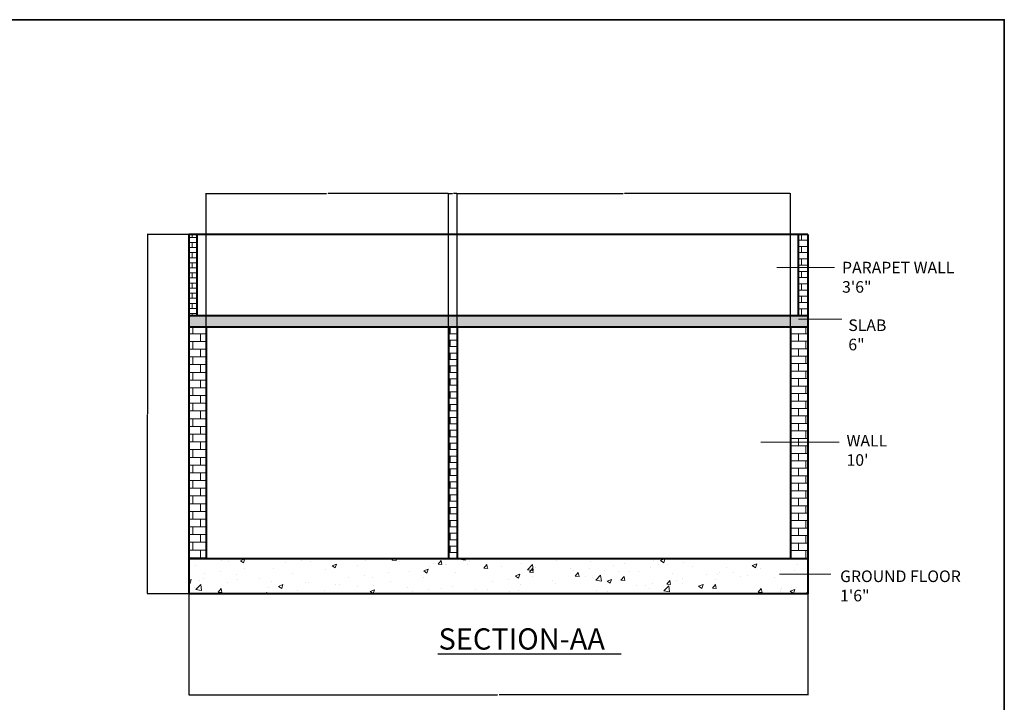
# Model space of a CAD drawing. Units: inches. Extents: x 1441 to 2460, y 1648 to 2683.
# Tile 35 of 35: x 1950 to 2460, y 2329 to 2683. Entities that reach past the tile are written whole.
import ezdxf

# ---------------------------------------------------------------- set-up
doc = ezdxf.new("R2010")
doc.units = ezdxf.units.IN
for name, color, linetype, lineweight in [('A-ANNO-DIMS', 2, 'Continuous', 18), ('A-ANNO-TEXT', 7, 'Continuous', 18), ('A-ANNO-TITL', 7, 'Continuous', 30), ('A-ANNO-TTLB', 7, 'Continuous', 35), ('A-SECT', 7, 'Continuous', 40)]:
    doc.layers.add(name, color=color, linetype=linetype, lineweight=lineweight)
doc.layers.add('A-SECT-PATT', color=251, linetype='Continuous', lineweight=13, true_color=0x636466)
doc.styles.get("Standard").update_dxf_attribs({"font": 'arial.ttf'})
doc.dimstyles.get("Standard").update_dxf_attribs({"dimtxt": 0.18, "dimasz": 0.18, "dimexe": 0.18, "dimexo": 0.0625, "dimgap": 0.09, "dimtad": 0, "dimtih": 1, "dimtoh": 1, "dimdec": 4, "dimzin": 0, "dimdsep": 46, "dimtxsty": 'Standard', "dimcen": 0.09, "dimadec": 0, "dimazin": 0, "dimtfac": 1, "dimtdec": 4, "dimtofl": 0, "dimtmove": 0, "dimatfit": 3, "dimfxl": 1, "dimtolj": 1, "dimtzin": 0, "dimarcsym": 0})

# ---------------------------------------------------------------- blocks, each defined once
blk = doc.blocks.new('*D119')
at = {"layer": 'A-ANNO-DIMS', "color": 0, "lineweight": -2, "transparency": 16777216}
for p, q in [((2037.9, 2385.3), (2037.9, 2332.77)), ((2358.4, 2385.3), (2358.4, 2332.77)), ((2038.08, 2332.95), (2197.76, 2332.95)), ((2358.22, 2332.95), (2198.55, 2332.95))]:
    blk.add_line(p, q, dxfattribs=at)
at = {"layer": 'A-ANNO-DIMS', "color": 0, "transparency": 16777216}
for points in [[(2038.08, 2332.98), (2038.08, 2332.92), (2037.9, 2332.95)], [(2358.22, 2332.98), (2358.22, 2332.92), (2358.4, 2332.95)]]:
    blk.add_solid(points, dxfattribs=at)
at = {"layer": 'Defpoints', "color": 0, "transparency": 16777216}
for p in [(2037.9, 2385.36), (2358.4, 2385.36), (2358.4, 2332.95)]:
    blk.add_point(p, dxfattribs=at)
at = {"layer": 'A-ANNO-DIMS', "color": 0, "transparency": 16777216, "insert": (2198.15, 2332.95), "char_height": 0.18, "attachment_point": 5}
blk.add_mtext('\\A1;320.5', dxfattribs=at)
blk = doc.blocks.new('*D120')
at = {"layer": 'A-ANNO-DIMS', "color": 0, "lineweight": -2, "transparency": 16777216}
for p, q in [((2037.84, 2571.36), (2016.37, 2571.36)), ((2016.55, 2571.18), (2016.55, 2478.54)), ((2016.55, 2385.54), (2016.55, 2478.18)), ((2037.84, 2385.36), (2016.37, 2385.36))]:
    blk.add_line(p, q, dxfattribs=at)
at = {"layer": 'A-ANNO-DIMS', "color": 0, "transparency": 16777216}
for points in [[(2016.52, 2571.18), (2016.58, 2571.18), (2016.55, 2571.36)], [(2016.52, 2385.54), (2016.58, 2385.54), (2016.55, 2385.36)]]:
    blk.add_solid(points, dxfattribs=at)
at = {"layer": 'Defpoints', "color": 0, "transparency": 16777216}
for p in [(2016.55, 2571.36), (2037.9, 2571.36), (2037.9, 2385.36)]:
    blk.add_point(p, dxfattribs=at)
at = {"layer": 'A-ANNO-DIMS', "color": 0, "transparency": 16777216, "insert": (2016.55, 2478.36), "char_height": 0.18, "attachment_point": 5}
blk.add_mtext('\\A1;186', dxfattribs=at)
blk = doc.blocks.new('*D121')
at = {"layer": 'A-ANNO-DIMS', "color": 0, "lineweight": -2, "transparency": 16777216}
for p, q in [((2046.9, 2523.42), (2046.9, 2592.89)), ((2047.08, 2592.71), (2109.27, 2592.71)), ((2172.22, 2592.71), (2110.04, 2592.71)), ((2172.4, 2523.42), (2172.4, 2592.89))]:
    blk.add_line(p, q, dxfattribs=at)
at = {"layer": 'A-ANNO-DIMS', "color": 0, "transparency": 16777216}
for points in [[(2047.08, 2592.74), (2047.08, 2592.68), (2046.9, 2592.71)], [(2172.22, 2592.74), (2172.22, 2592.68), (2172.4, 2592.71)]]:
    blk.add_solid(points, dxfattribs=at)
at = {"layer": 'Defpoints', "color": 0, "transparency": 16777216}
for p in [(2172.4, 2592.71), (2046.9, 2523.36), (2172.4, 2523.36)]:
    blk.add_point(p, dxfattribs=at)
at = {"layer": 'A-ANNO-DIMS', "color": 0, "transparency": 16777216, "insert": (2109.65, 2592.71), "char_height": 0.18, "attachment_point": 5}
blk.add_mtext('\\A1;125.5', dxfattribs=at)
blk = doc.blocks.new('*D122')
at = {"layer": 'A-ANNO-DIMS', "color": 0, "lineweight": -2, "transparency": 16777216}
for p, q in [((2172.4, 2523.42), (2172.4, 2592.89)), ((2172.58, 2592.71), (2174.39, 2592.71)), ((2176.72, 2592.71), (2174.91, 2592.71)), ((2176.9, 2523.42), (2176.9, 2592.89))]:
    blk.add_line(p, q, dxfattribs=at)
at = {"layer": 'A-ANNO-DIMS', "color": 0, "transparency": 16777216}
for points in [[(2172.58, 2592.74), (2172.58, 2592.68), (2172.4, 2592.71)], [(2176.72, 2592.74), (2176.72, 2592.68), (2176.9, 2592.71)]]:
    blk.add_solid(points, dxfattribs=at)
at = {"layer": 'Defpoints', "color": 0, "transparency": 16777216}
for p in [(2176.9, 2592.71), (2172.4, 2523.36), (2176.9, 2523.36)]:
    blk.add_point(p, dxfattribs=at)
at = {"layer": 'A-ANNO-DIMS', "color": 0, "transparency": 16777216, "insert": (2174.65, 2592.71), "char_height": 0.18, "attachment_point": 5}
blk.add_mtext('\\A1;4.5', dxfattribs=at)
blk = doc.blocks.new('*D123')
at = {"layer": 'A-ANNO-DIMS', "color": 0, "lineweight": -2, "transparency": 16777216}
for p, q in [((2176.9, 2523.42), (2176.9, 2592.89)), ((2177.08, 2592.71), (2262.77, 2592.71)), ((2349.22, 2592.71), (2263.54, 2592.71)), ((2349.4, 2523.42), (2349.4, 2592.89))]:
    blk.add_line(p, q, dxfattribs=at)
at = {"layer": 'A-ANNO-DIMS', "color": 0, "transparency": 16777216}
for points in [[(2177.08, 2592.74), (2177.08, 2592.68), (2176.9, 2592.71)], [(2349.22, 2592.74), (2349.22, 2592.68), (2349.4, 2592.71)]]:
    blk.add_solid(points, dxfattribs=at)
at = {"layer": 'Defpoints', "color": 0, "transparency": 16777216}
for p in [(2349.4, 2592.71), (2176.9, 2523.36), (2349.4, 2523.36)]:
    blk.add_point(p, dxfattribs=at)
at = {"layer": 'A-ANNO-DIMS', "color": 0, "transparency": 16777216, "insert": (2263.15, 2592.71), "char_height": 0.18, "attachment_point": 5}
blk.add_mtext('\\A1;172.5', dxfattribs=at)

msp = doc.modelspace()

# ---------------------------------------------------------------- hatches: boundary and pattern name
at = {"layer": 'A-SECT-PATT'}
h = msp.add_hatch(dxfattribs=at)
h.set_pattern_fill('BRICK', color=256, scale=0.413386, style=0)
h.paths.add_polyline_path([(2037.9015, 2529.3623), (2042.3172, 2529.3623), (2042.3172, 2571.3623), (2037.9015, 2571.3623)])
h = msp.add_hatch(dxfattribs=at)
h.set_pattern_fill('BRICK', color=256, scale=0.508783, style=0)
h.paths.add_polyline_path([(2353.6639, 2529.3623), (2358.4015, 2529.3623), (2358.4015, 2571.3623), (2353.6639, 2571.3623)])
at = {"layer": 'A-SECT-PATT', "transparency": 33554587}
h = msp.add_hatch(color=256, dxfattribs=at)
h.dxf.hatch_style = 1
h.paths.add_polyline_path([(2358.4015, 2529.3623), (2037.9015, 2529.3623), (2037.9015, 2523.3623), (2358.4015, 2523.3623)])
at = {"layer": 'A-SECT-PATT'}
h = msp.add_hatch(dxfattribs=at)
h.set_pattern_fill('BRICK', color=256, scale=0.629921, style=0)
h.paths.add_polyline_path([(2037.9015, 2403.3623), (2046.9015, 2403.3623), (2046.9015, 2523.3623), (2037.9015, 2523.3623)])
h = msp.add_hatch(dxfattribs=at)
h.set_pattern_fill('BRICK', color=256, scale=0.524934, style=0)
h.paths.add_polyline_path([(2172.4015, 2403.3623), (2176.9015, 2403.3623), (2176.9015, 2523.3623), (2172.4015, 2523.3623)])
h = msp.add_hatch(dxfattribs=at)
h.set_pattern_fill('BRICK', color=256, scale=0.609601, style=0)
h.paths.add_polyline_path([(2349.4015, 2403.3623), (2358.4015, 2403.3623), (2358.4015, 2523.3623), (2349.4015, 2523.3623)])
h = msp.add_hatch(dxfattribs=at)
h.set_pattern_fill('AR-CONC', color=256, scale=0.13, style=0)
h.paths.add_polyline_path([(2037.9015, 2385.3623), (2358.4015, 2385.3623), (2358.4015, 2403.3623), (2037.9015, 2403.3623)])

# ---------------------------------------------------------------- linework, layer by layer
at = {"layer": 'A-ANNO-TEXT'}
for p, q in [((2342.4553, 2554.3663), (2372.217, 2554.3663)), ((2353.6294, 2527.5199), (2376.1382, 2527.5199)), ((2334.1361, 2463.8826), (2374.7485, 2463.8826)), ((2343.8605, 2395.5812), (2370.3371, 2395.5812))]:
    msp.add_line(p, q, dxfattribs=at)
at = {"layer": 'A-ANNO-TITL'}
msp.add_line((2166.8437, 2354.299), (2261.7625, 2354.299), dxfattribs=at)
at = {"layer": 'A-ANNO-TTLB'}
msp.add_lwpolyline([(1440.5107, 2682.6413), (2460.193, 2682.6413), (2460.193, 1648.08), (1440.5107, 1648.08)], close=True, dxfattribs=at)
at = {"layer": 'A-SECT'}
for p, q in [((2037.9015, 2571.3623), (2037.9015, 2385.3623)), ((2358.4015, 2571.3623), (2037.9015, 2571.3623)), ((2042.3172, 2529.3623), (2042.3172, 2571.3623)), ((2353.6639, 2529.3623), (2353.6639, 2571.3623)), ((2358.4015, 2571.3623), (2358.4015, 2385.3623)), ((2358.4015, 2529.3623), (2037.9015, 2529.3623)), ((2358.4015, 2523.3623), (2037.9015, 2523.3623)), ((2046.9015, 2523.3623), (2046.9015, 2403.3623)), ((2172.4015, 2523.3623), (2172.4015, 2403.3623)), ((2176.9015, 2523.3623), (2176.9015, 2403.3623)), ((2349.4015, 2523.3623), (2349.4015, 2403.3623)), ((2358.4015, 2403.3623), (2037.9015, 2403.3623)), ((2358.4015, 2385.3623), (2037.9015, 2385.3623))]:
    msp.add_line(p, q, dxfattribs=at)

# ---------------------------------------------------------------- texts
at = {"layer": 'A-ANNO-TEXT', "char_height": 6, "attachment_point": 1}
for s, width, insert in [('PARAPET WALL\\P3\'6"', 65.191636, (2376.1775, 2557.2637)), ('SLAB\\P6"', 65.563617, (2379.4325, 2527.4236)), ("WALL\\P10'", 81.698306, (2378.4947, 2467.6229)), ('GROUND FLOOR\\P1\'6"', 85.037404, (2375.1556, 2397.4159))]:
    msp.add_mtext_dynamic_manual_height_columns(s, width=width, gutter_width=12.5, heights=[0], dxfattribs=dict(at, insert=insert))
at = {"layer": 'A-ANNO-TITL', "insert": (2167.2302, 2367.4435), "char_height": 11, "attachment_point": 1}
msp.add_mtext_dynamic_manual_height_columns('SECTION-AA', width=230.745998, gutter_width=12.5, heights=[0], dxfattribs=at)

# ---------------------------------------------------------------- dimensions: what is measured, and where the dimension line sits
at = {"layer": 'A-ANNO-DIMS'}
for base, p1, p2, picture, middle in [((2172.4015, 2592.7123), (2046.9015, 2523.3623), (2172.4015, 2523.3623), '*D121', (2109.6515, 2592.7123)), ((2176.9015, 2592.7123), (2172.4015, 2523.3623), (2176.9015, 2523.3623), '*D122', (2174.6515, 2592.7123)), ((2349.4015, 2592.7123), (2176.9015, 2523.3623), (2349.4015, 2523.3623), '*D123', (2263.1515, 2592.7123)), ((2358.4015, 2332.949), (2037.9015, 2385.3623), (2358.4015, 2385.3623), '*D119', (2198.1515, 2332.949))]:
    dim = msp.add_linear_dim(base=base, p1=p1, p2=p2, dimstyle='Standard', override={"dimdec": 1, "dimlfac": 1, "dimrnd": 0, "dimzin": 0, "dimdsep": 46, "dimlunit": 2}, dxfattribs=at)
    dim.commit()
    dim.dimension.update_dxf_attribs({"geometry": picture, "text_midpoint": middle})
dim = msp.add_linear_dim(base=(2016.5515, 2571.3623), p1=(2037.9015, 2385.3623), p2=(2037.9015, 2571.3623), angle=90, dimstyle='Standard', override={"dimdec": 0, "dimlfac": 1, "dimrnd": 0, "dimzin": 0, "dimdsep": 46, "dimlunit": 2}, dxfattribs=at)
dim.commit()
dim.dimension.update_dxf_attribs({"geometry": '*D120', "text_midpoint": (2016.5515, 2478.3623)})

doc.saveas('drawing.dxf')
